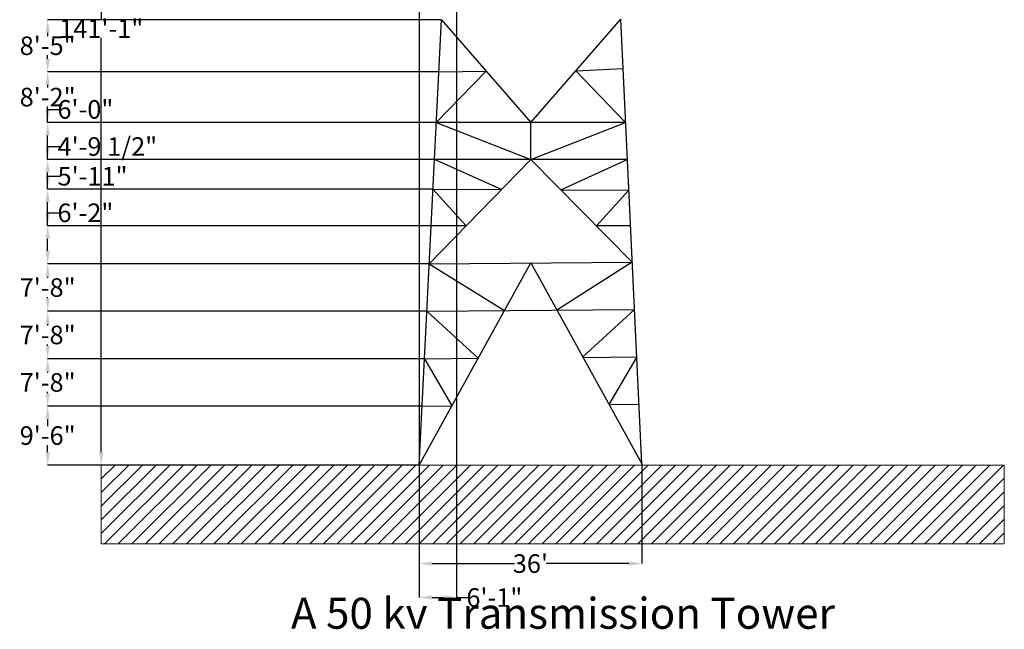
# Model space of a CAD drawing. Units: inches. Extents: x -827 to 1185, y -311 to 1858.
# Tile 1 of 2: x -754 to 1156, y -311 to 871. Entities that reach past the tile are written whole.
import ezdxf

# ---------------------------------------------------------------- set-up
doc = ezdxf.new("R2010")
doc.units = ezdxf.units.IN
doc.header["$MEASUREMENT"] = 0
for name, color, linetype, lineweight in [('C-TOPO-PATT', 8, 'Continuous', 18), ('S-ANNO-DIMS', 2, 'Continuous', 18), ('S-ANNO-TEXT', 7, 'Continuous', 25), ('S-TOWR', 5, 'Continuous', 30)]:
    doc.layers.add(name, color=color, linetype=linetype, lineweight=lineweight)
doc.styles.get("Standard").update_dxf_attribs({"font": 'arial.ttf'})
doc.dimstyles.get("Standard").update_dxf_attribs({"dimtxt": 36, "dimasz": 25.18, "dimexe": 0.18, "dimexo": 0.0625, "dimgap": 0.09, "dimtad": 0, "dimtih": 1, "dimtoh": 1, "dimdec": 0, "dimzin": 0, "dimdsep": 46, "dimlunit": 3, "dimtxsty": 'Standard', "dimcen": 0.09, "dimclrd": 4, "dimadec": 0, "dimazin": 0, "dimtfac": 1, "dimtdec": 0, "dimtofl": 0, "dimtmove": 0, "dimatfit": 3, "dimfxl": 1, "dimtolj": 1, "dimtzin": 0, "dimarcsym": 0})

# ---------------------------------------------------------------- blocks, each defined once
blk = doc.blocks.new('*D1')
at = {"layer": 'Defpoints', "color": 0, "transparency": 16777216}
for p in [(20.6, 7.5), (452.6, 9.7), (452.6, -183.7)]:
    blk.add_point(p, dxfattribs=at)
at = {"layer": 'S-ANNO-DIMS', "color": 0, "lineweight": -2, "transparency": 16777216}
for p, q in [((20.6, 7.4), (20.6, -183.8)), ((452.6, 9.6), (452.6, -183.8)), ((45.8, -183.7), (206, -183.7)), ((427.4, -183.7), (267.2, -183.7))]:
    blk.add_line(p, q, dxfattribs=at)
at = {"layer": 'S-ANNO-DIMS', "color": 0, "transparency": 16777216}
for points in [[(45.8, -179.5), (45.8, -187.9), (20.6, -183.7)], [(427.4, -179.5), (427.4, -187.9), (452.6, -183.7)]]:
    blk.add_solid(points, dxfattribs=at)
at = {"layer": 'S-ANNO-DIMS', "color": 0, "transparency": 16777216, "insert": (236.6, -183.7), "char_height": 36, "attachment_point": 5}
blk.add_mtext("\\A1;36'", dxfattribs=at)
blk = doc.blocks.new('*D6')
at = {"layer": 'Defpoints', "color": 0, "transparency": 16777216}
for p in [(-159.4, 1700.6), (-595.9, 7.5), (20.6, 7.5)]:
    blk.add_point(p, dxfattribs=at)
at = {"layer": 'S-ANNO-DIMS', "color": 0, "lineweight": -2, "transparency": 16777216}
for p, q in [((-159.5, 1700.6), (-596.1, 1700.6)), ((-595.9, 1675.4), (-595.9, 872.2)), ((-595.9, 32.6), (-595.9, 835.9)), ((20.5, 7.5), (-596.1, 7.5))]:
    blk.add_line(p, q, dxfattribs=at)
at = {"layer": 'S-ANNO-DIMS', "color": 0, "transparency": 16777216}
for points in [[(-600.1, 1675.4), (-591.7, 1675.4), (-595.9, 1700.6)], [(-600.1, 32.6), (-591.7, 32.6), (-595.9, 7.5)]]:
    blk.add_solid(points, dxfattribs=at)
at = {"layer": 'S-ANNO-DIMS', "color": 0, "transparency": 16777216, "insert": (-595.9, 854), "char_height": 36, "attachment_point": 5}
blk.add_mtext('\\A1;141\'-1"', dxfattribs=at)
blk = doc.blocks.new('*D15')
at = {"layer": 'Defpoints', "color": 0, "transparency": 16777216}
for p in [(-699.9, 121.7), (26.3, 121.7), (20.6, 7.5)]:
    blk.add_point(p, dxfattribs=at)
at = {"layer": 'S-ANNO-DIMS', "color": 0, "lineweight": -2, "transparency": 16777216}
for p, q in [((26.2, 121.7), (-700.1, 121.7)), ((20.5, 7.5), (-700.1, 7.5))]:
    blk.add_line(p, q, dxfattribs=at)
at = {"layer": 'S-ANNO-DIMS', "color": 4, "lineweight": -2, "transparency": 16777216}
for p, q in [((-699.9, 96.5), (-699.9, 83)), ((-699.9, 32.6), (-699.9, 46.1))]:
    blk.add_line(p, q, dxfattribs=at)
at = {"layer": 'S-ANNO-DIMS', "color": 4, "transparency": 16777216}
for points in [[(-704.1, 96.5), (-695.7, 96.5), (-699.9, 121.7)], [(-704.1, 32.6), (-695.7, 32.6), (-699.9, 7.5)]]:
    blk.add_solid(points, dxfattribs=at)
at = {"layer": 'S-ANNO-DIMS', "color": 0, "transparency": 16777216, "insert": (-699.9, 64.6), "char_height": 36, "attachment_point": 5}
blk.add_mtext('\\A1;9\'-6"', dxfattribs=at)
blk = doc.blocks.new('*D16')
at = {"layer": 'Defpoints', "color": 0, "transparency": 16777216}
for p in [(-699.9, 213.7), (30.9, 213.7), (26.3, 121.7)]:
    blk.add_point(p, dxfattribs=at)
at = {"layer": 'S-ANNO-DIMS', "color": 0, "lineweight": -2, "transparency": 16777216}
for p, q in [((30.9, 213.7), (-700.1, 213.7)), ((26.2, 121.7), (-700.1, 121.7))]:
    blk.add_line(p, q, dxfattribs=at)
at = {"layer": 'S-ANNO-DIMS', "color": 4, "lineweight": -2, "transparency": 16777216}
for p, q in [((-699.9, 188.5), (-699.9, 186.2)), ((-699.9, 146.8), (-699.9, 149.2))]:
    blk.add_line(p, q, dxfattribs=at)
at = {"layer": 'S-ANNO-DIMS', "color": 4, "transparency": 16777216}
for points in [[(-704.1, 188.5), (-695.7, 188.5), (-699.9, 213.7)], [(-704.1, 146.8), (-695.7, 146.8), (-699.9, 121.7)]]:
    blk.add_solid(points, dxfattribs=at)
at = {"layer": 'S-ANNO-DIMS', "color": 0, "transparency": 16777216, "insert": (-699.9, 167.7), "char_height": 36, "attachment_point": 5}
blk.add_mtext('\\A1;7\'-8"', dxfattribs=at)
blk = doc.blocks.new('*D17')
at = {"layer": 'Defpoints', "color": 0, "transparency": 16777216}
for p in [(-699.9, 305.8), (35.5, 305.8), (30.9, 213.7)]:
    blk.add_point(p, dxfattribs=at)
at = {"layer": 'S-ANNO-DIMS', "color": 0, "lineweight": -2, "transparency": 16777216}
for p, q in [((35.5, 305.8), (-700.1, 305.8)), ((30.9, 213.7), (-700.1, 213.7))]:
    blk.add_line(p, q, dxfattribs=at)
at = {"layer": 'S-ANNO-DIMS', "color": 4, "lineweight": -2, "transparency": 16777216}
for p, q in [((-699.9, 280.6), (-699.9, 278.2)), ((-699.9, 238.9), (-699.9, 241.3))]:
    blk.add_line(p, q, dxfattribs=at)
at = {"layer": 'S-ANNO-DIMS', "color": 4, "transparency": 16777216}
for points in [[(-704.1, 280.6), (-695.7, 280.6), (-699.9, 305.8)], [(-704.1, 238.9), (-695.7, 238.9), (-699.9, 213.7)]]:
    blk.add_solid(points, dxfattribs=at)
at = {"layer": 'S-ANNO-DIMS', "color": 0, "transparency": 16777216, "insert": (-699.9, 259.8), "char_height": 36, "attachment_point": 5}
blk.add_mtext('\\A1;7\'-8"', dxfattribs=at)
blk = doc.blocks.new('*D18')
at = {"layer": 'Defpoints', "color": 0, "transparency": 16777216}
for p in [(-699.9, 397.8), (40.2, 397.8), (35.5, 305.8)]:
    blk.add_point(p, dxfattribs=at)
at = {"layer": 'S-ANNO-DIMS', "color": 0, "lineweight": -2, "transparency": 16777216}
for p, q in [((40.1, 397.8), (-700.1, 397.8)), ((35.5, 305.8), (-700.1, 305.8))]:
    blk.add_line(p, q, dxfattribs=at)
at = {"layer": 'S-ANNO-DIMS', "color": 4, "lineweight": -2, "transparency": 16777216}
for p, q in [((-699.9, 372.7), (-699.9, 370.3)), ((-699.9, 331), (-699.9, 333.3))]:
    blk.add_line(p, q, dxfattribs=at)
at = {"layer": 'S-ANNO-DIMS', "color": 4, "transparency": 16777216}
for points in [[(-704.1, 372.7), (-695.7, 372.7), (-699.9, 397.8)], [(-704.1, 331), (-695.7, 331), (-699.9, 305.8)]]:
    blk.add_solid(points, dxfattribs=at)
at = {"layer": 'S-ANNO-DIMS', "color": 0, "transparency": 16777216, "insert": (-699.9, 351.8), "char_height": 36, "attachment_point": 5}
blk.add_mtext('\\A1;7\'-8"', dxfattribs=at)
blk = doc.blocks.new('*D19')
at = {"layer": 'Defpoints', "color": 0, "transparency": 16777216}
for p in [(-699.9, 471.6), (44.9, 471.6), (40.2, 397.8)]:
    blk.add_point(p, dxfattribs=at)
at = {"layer": 'S-ANNO-DIMS', "color": 4, "lineweight": -2, "transparency": 16777216}
for p, q in [((-699.9, 471.6), (-699.9, 496.8)), ((-699.9, 496.8), (-674.7, 496.8)), ((-699.9, 423), (-699.9, 446.5))]:
    blk.add_line(p, q, dxfattribs=at)
at = {"layer": 'S-ANNO-DIMS', "color": 0, "lineweight": -2, "transparency": 16777216}
for p, q in [((44.8, 471.6), (-700.1, 471.6)), ((40.1, 397.8), (-700.1, 397.8))]:
    blk.add_line(p, q, dxfattribs=at)
at = {"layer": 'S-ANNO-DIMS', "color": 4, "transparency": 16777216}
for points in [[(-704.1, 446.5), (-695.7, 446.5), (-699.9, 471.6)], [(-704.1, 423), (-695.7, 423), (-699.9, 397.8)]]:
    blk.add_solid(points, dxfattribs=at)
at = {"layer": 'S-ANNO-DIMS', "color": 0, "transparency": 16777216, "insert": (-626.7, 496.8), "char_height": 36, "attachment_point": 5}
blk.add_mtext('\\A1;6\'-2"', dxfattribs=at)
blk = doc.blocks.new('*D20')
at = {"layer": 'Defpoints', "color": 0, "transparency": 16777216}
for p in [(-699.9, 542.5), (47.4, 542.5), (44.9, 471.6)]:
    blk.add_point(p, dxfattribs=at)
at = {"layer": 'S-ANNO-DIMS', "color": 4, "lineweight": -2, "transparency": 16777216}
for p, q in [((-699.9, 542.5), (-699.9, 567.7)), ((-699.9, 567.7), (-674.7, 567.7)), ((-699.9, 496.8), (-699.9, 517.3))]:
    blk.add_line(p, q, dxfattribs=at)
at = {"layer": 'S-ANNO-DIMS', "color": 0, "lineweight": -2, "transparency": 16777216}
for p, q in [((47.4, 542.5), (-700.1, 542.5)), ((44.8, 471.6), (-700.1, 471.6))]:
    blk.add_line(p, q, dxfattribs=at)
at = {"layer": 'S-ANNO-DIMS', "color": 4, "transparency": 16777216}
for points in [[(-704.1, 517.3), (-695.7, 517.3), (-699.9, 542.5)], [(-704.1, 496.8), (-695.7, 496.8), (-699.9, 471.6)]]:
    blk.add_solid(points, dxfattribs=at)
at = {"layer": 'S-ANNO-DIMS', "color": 0, "transparency": 16777216, "insert": (-612.8, 567.7), "char_height": 36, "attachment_point": 5}
blk.add_mtext('\\A1;5\'-11"', dxfattribs=at)
blk = doc.blocks.new('*D21')
at = {"layer": 'Defpoints', "color": 0, "transparency": 16777216}
for p in [(-699.9, 600.2), (50.9, 600.2), (47.4, 542.5)]:
    blk.add_point(p, dxfattribs=at)
at = {"layer": 'S-ANNO-DIMS', "color": 4, "lineweight": -2, "transparency": 16777216}
for p, q in [((-699.9, 600.2), (-699.9, 625.3)), ((-699.9, 625.3), (-674.7, 625.3)), ((-699.9, 567.7), (-699.9, 575))]:
    blk.add_line(p, q, dxfattribs=at)
at = {"layer": 'S-ANNO-DIMS', "color": 0, "lineweight": -2, "transparency": 16777216}
for p, q in [((50.8, 600.2), (-700.1, 600.2)), ((47.4, 542.5), (-700.1, 542.5))]:
    blk.add_line(p, q, dxfattribs=at)
at = {"layer": 'S-ANNO-DIMS', "color": 4, "transparency": 16777216}
for points in [[(-704.1, 575), (-695.7, 575), (-699.9, 600.2)], [(-704.1, 567.7), (-695.7, 567.7), (-699.9, 542.5)]]:
    blk.add_solid(points, dxfattribs=at)
at = {"layer": 'S-ANNO-DIMS', "color": 0, "transparency": 16777216, "insert": (-584.1, 625.3), "char_height": 36, "attachment_point": 5}
blk.add_mtext('\\A1;4\'-9 1/2"', dxfattribs=at)
blk = doc.blocks.new('*D22')
at = {"layer": 'Defpoints', "color": 0, "transparency": 16777216}
for p in [(-699.9, 672.2), (53.9, 672.2), (50.9, 600.2)]:
    blk.add_point(p, dxfattribs=at)
at = {"layer": 'S-ANNO-DIMS', "color": 4, "lineweight": -2, "transparency": 16777216}
for p, q in [((-699.9, 672.2), (-699.9, 697.4)), ((-699.9, 697.4), (-674.7, 697.4)), ((-699.9, 625.3), (-699.9, 647))]:
    blk.add_line(p, q, dxfattribs=at)
at = {"layer": 'S-ANNO-DIMS', "color": 0, "lineweight": -2, "transparency": 16777216}
for p, q in [((53.9, 672.2), (-700.1, 672.2)), ((50.8, 600.2), (-700.1, 600.2))]:
    blk.add_line(p, q, dxfattribs=at)
at = {"layer": 'S-ANNO-DIMS', "color": 4, "transparency": 16777216}
for points in [[(-704.1, 647), (-695.7, 647), (-699.9, 672.2)], [(-704.1, 625.3), (-695.7, 625.3), (-699.9, 600.2)]]:
    blk.add_solid(points, dxfattribs=at)
at = {"layer": 'S-ANNO-DIMS', "color": 0, "transparency": 16777216, "insert": (-626.7, 697.4), "char_height": 36, "attachment_point": 5}
blk.add_mtext('\\A1;6\'-0"', dxfattribs=at)
blk = doc.blocks.new('*D23')
at = {"layer": 'Defpoints', "color": 0, "transparency": 16777216}
for p in [(-699.9, 770.1), (58.8, 770.1), (53.9, 672.2)]:
    blk.add_point(p, dxfattribs=at)
at = {"layer": 'S-ANNO-DIMS', "color": 0, "lineweight": -2, "transparency": 16777216}
for p, q in [((58.8, 770.1), (-700.1, 770.1)), ((53.9, 672.2), (-700.1, 672.2))]:
    blk.add_line(p, q, dxfattribs=at)
at = {"layer": 'S-ANNO-DIMS', "color": 4, "lineweight": -2, "transparency": 16777216}
for p, q in [((-699.9, 745), (-699.9, 739.7)), ((-699.9, 697.4), (-699.9, 702.7))]:
    blk.add_line(p, q, dxfattribs=at)
at = {"layer": 'S-ANNO-DIMS', "color": 4, "transparency": 16777216}
for points in [[(-704.1, 745), (-695.7, 745), (-699.9, 770.1)], [(-704.1, 697.4), (-695.7, 697.4), (-699.9, 672.2)]]:
    blk.add_solid(points, dxfattribs=at)
at = {"layer": 'S-ANNO-DIMS', "color": 0, "transparency": 16777216, "insert": (-699.9, 721.2), "char_height": 36, "attachment_point": 5}
blk.add_mtext('\\A1;8\'-2"', dxfattribs=at)
blk = doc.blocks.new('*D24')
at = {"layer": 'Defpoints', "color": 0, "transparency": 16777216}
for p in [(-699.9, 871.4), (63.9, 871.4), (58.8, 770.1)]:
    blk.add_point(p, dxfattribs=at)
at = {"layer": 'S-ANNO-DIMS', "color": 0, "lineweight": -2, "transparency": 16777216}
for p, q in [((63.8, 871.4), (-700.1, 871.4)), ((58.8, 770.1), (-700.1, 770.1))]:
    blk.add_line(p, q, dxfattribs=at)
at = {"layer": 'S-ANNO-DIMS', "color": 4, "lineweight": -2, "transparency": 16777216}
for p, q in [((-699.9, 846.2), (-699.9, 839.2)), ((-699.9, 795.3), (-699.9, 802.3))]:
    blk.add_line(p, q, dxfattribs=at)
at = {"layer": 'S-ANNO-DIMS', "color": 4, "transparency": 16777216}
for points in [[(-704.1, 846.2), (-695.7, 846.2), (-699.9, 871.4)], [(-704.1, 795.3), (-695.7, 795.3), (-699.9, 770.1)]]:
    blk.add_solid(points, dxfattribs=at)
at = {"layer": 'S-ANNO-DIMS', "color": 0, "transparency": 16777216, "insert": (-699.9, 820.8), "char_height": 36, "attachment_point": 5}
blk.add_mtext('\\A1;8\'-5"', dxfattribs=at)
blk = doc.blocks.new('*D33')
at = {"layer": 'Defpoints', "color": 0, "transparency": 16777216}
for p in [(20.6, 1496.6), (93.5, 1496.6), (93.5, -249.5)]:
    blk.add_point(p, dxfattribs=at)
at = {"layer": 'S-ANNO-DIMS', "color": 0, "lineweight": -2, "transparency": 16777216}
for p, q in [((20.6, 1496.5), (20.6, -249.7)), ((93.5, 1496.5), (93.5, -249.7))]:
    blk.add_line(p, q, dxfattribs=at)
at = {"layer": 'S-ANNO-DIMS', "color": 4, "lineweight": -2, "transparency": 16777216}
for p, q in [((45.8, -249.5), (68.3, -249.5)), ((93.5, -249.5), (118.7, -249.5))]:
    blk.add_line(p, q, dxfattribs=at)
at = {"layer": 'S-ANNO-DIMS', "color": 4, "transparency": 16777216}
for points in [[(45.8, -245.3), (45.8, -253.7), (20.6, -249.5)], [(68.3, -245.3), (68.3, -253.7), (93.5, -249.5)]]:
    blk.add_solid(points, dxfattribs=at)
at = {"layer": 'S-ANNO-DIMS', "color": 0, "transparency": 16777216, "insert": (166.7, -249.5), "char_height": 36, "attachment_point": 5}
blk.add_mtext('\\A1;6\'-1"', dxfattribs=at)

msp = doc.modelspace()

# ---------------------------------------------------------------- hatches: boundary and pattern name
at = {"layer": 'C-TOPO-PATT'}
h = msp.add_hatch(dxfattribs=at)
h.set_pattern_fill('ANSI31', color=256, scale=150, style=0)
h.set_pattern_definition([(45, (-1783.912, -146.804), (-13.25825, 13.25825), [])])
h.paths.add_polyline_path([(-595.91, 7.45), (1155.95, 7.45), (1155.95, -145.49), (-595.91, -145.49)])

# ---------------------------------------------------------------- linework, layer by layer
msp.add_lwpolyline([(-595.91, 7.45), (1155.95, 7.45), (1155.95, -145.49), (-595.91, -145.49)], close=True, dxfattribs=at)
at = {"layer": 'S-TOWR'}
for p, q in [((20.58, 7.45), (63.91, 871.37)), ((63.91, 871.37), (237.6, 672.23)), ((237.6, 672.23), (411.9, 872.2)), ((452.58, 9.7), (411.9, 872.2)), ((53.92, 672.23), (150.75, 771.8)), ((58.83, 770.15), (150.75, 771.8)), ((324.37, 772.06), (324.11, 772.06)), ((324.37, 772.06), (324.24, 772.21)), ((324.75, 772.22), (416.41, 776.54)), ((421.33, 672.23), (324.75, 772.22)), ((421.33, 672.23), (53.92, 672.23)), ((53.92, 672.23), (237.51, 600.15)), ((236.58, 672.23), (238, 672.69)), ((239.29, 672.25), (236.58, 672.23)), ((237.48, 672.24), (238.38, 672.24)), ((237.49, 600.15), (237.6, 672.56)), ((237.51, 600.15), (421.33, 672.23)), ((237.49, 600.15), (40.16, 397.85)), ((424.11, 600.15), (50.87, 600.15)), ((181.61, 541.24), (50.87, 600.15)), ((237.49, 600.16), (434.11, 401.2)), ((295.71, 541.24), (424.11, 600.15)), ((47.42, 542.5), (47.38, 542.26)), ((47.38, 542.26), (47.41, 542.26)), ((112.14, 471.64), (47.42, 542.5)), ((47.42, 542.5), (180.6, 541.83)), ((295.71, 541.24), (427.54, 540.58)), ((427.54, 540.58), (364.5, 471.64)), ((427.06, 541.38), (426.99, 541.38)), ((112.14, 471.64), (44.87, 471.64)), ((429.78, 471.64), (364.5, 471.64)), ((40.16, 397.85), (434.11, 401.2)), ((434.11, 401.2), (287.79, 307.93)), ((20.58, 7.45), (237.18, 399.52)), ((40.16, 397.85), (186.1, 307.06)), ((237.18, 399.52), (452.58, 9.7)), ((35.55, 305.78), (438.45, 309.21)), ((35.55, 305.78), (135.02, 214.6)), ((438.45, 309.21), (337.82, 216.67)), ((30.93, 213.72), (135.02, 214.6)), ((30.93, 213.72), (83.94, 122.14)), ((338.4, 216.33), (442.79, 217.22)), ((442.79, 217.22), (389.01, 124.74)), ((26.31, 121.65), (83.94, 122.14)), ((389.01, 124.74), (447.13, 125.23))]:
    msp.add_line(p, q, dxfattribs=at)

# ---------------------------------------------------------------- texts
at = {"layer": 'S-ANNO-TEXT', "insert": (-227.93, -250.13), "char_height": 60, "attachment_point": 1}
msp.add_mtext_dynamic_manual_height_columns('{A 50 kv Transmission Tower}', width=1214.4183, gutter_width=1, heights=[0], dxfattribs=at)

# ---------------------------------------------------------------- dimensions: what is measured, and where the dimension line sits
at = {"layer": 'S-ANNO-DIMS'}
for base, p1, p2, override, picture, middle in [((-595.91, 7.45), (-159.42, 1700.58), (20.58, 7.45), {"dimclrd": 0, "dimclre": 0, "dimclrt": 0}, '*D6', (-595.91, 854.01)), ((-699.91, 871.37), (58.83, 770.15), (63.91, 871.37), {"dimdec": 1, "dimlfac": 1, "dimrnd": 0, "dimzin": 1, "dimdsep": 46, "dimlunit": 4, "dimfrac": 2}, '*D24', (-699.91, 820.76)), ((-699.91, 770.15), (53.92, 672.23), (58.83, 770.15), {"dimdec": 1, "dimlfac": 1, "dimrnd": 0, "dimzin": 1, "dimdsep": 46, "dimlunit": 4, "dimfrac": 2}, '*D23', (-699.91, 721.19)), ((-699.91, 672.23), (50.87, 600.15), (53.92, 672.23), {"dimdec": 1, "dimlfac": 1, "dimrnd": 0, "dimzin": 1, "dimdsep": 46, "dimlunit": 4, "dimfrac": 2}, '*D22', (-626.7, 697.41)), ((-699.9144, 600.1522), (47.4176, 542.5024), (50.872, 600.1522), {"dimdec": 1, "dimlfac": 1, "dimrnd": 0, "dimzin": 1, "dimdsep": 46, "dimlunit": 4, "dimfrac": 2}, '*D21', (-584.1287, 625.3322)), ((-699.91, 542.5), (44.87, 471.64), (47.42, 542.5), {"dimdec": 1, "dimlfac": 1, "dimrnd": 0, "dimzin": 1, "dimdsep": 46, "dimlunit": 4, "dimfrac": 2}, '*D20', (-612.81, 567.68)), ((-699.91, 471.64), (40.16, 397.85), (44.87, 471.64), {"dimdec": 1, "dimlfac": 1, "dimrnd": 0, "dimzin": 1, "dimdsep": 46, "dimlunit": 4, "dimfrac": 2}, '*D19', (-626.7, 496.82)), ((-699.91, 397.85), (35.55, 305.78), (40.16, 397.85), {"dimdec": 1, "dimlfac": 1, "dimrnd": 0, "dimzin": 1, "dimdsep": 46, "dimlunit": 4, "dimfrac": 2}, '*D18', (-699.91, 351.81)), ((-699.91, 305.78), (30.93, 213.72), (35.55, 305.78), {"dimdec": 1, "dimlfac": 1, "dimrnd": 0, "dimzin": 1, "dimdsep": 46, "dimlunit": 4, "dimfrac": 2}, '*D17', (-699.91, 259.75)), ((-699.91, 213.72), (26.31, 121.65), (30.93, 213.72), {"dimdec": 1, "dimlfac": 1, "dimrnd": 0, "dimzin": 1, "dimdsep": 46, "dimlunit": 4, "dimfrac": 2}, '*D16', (-699.91, 167.69)), ((-699.91, 121.65), (20.58, 7.45), (26.31, 121.65), {"dimdec": 1, "dimlfac": 1, "dimrnd": 0, "dimzin": 1, "dimdsep": 46, "dimlunit": 4, "dimfrac": 2}, '*D15', (-699.91, 64.55))]:
    dim = msp.add_linear_dim(base=base, p1=p1, p2=p2, angle=90, dimstyle='Standard', override=override, dxfattribs=at)
    dim.commit()
    dim.dimension.update_dxf_attribs({"geometry": picture, "text_midpoint": middle})
for base, p1, p2, override, picture, middle in [((93.47, -249.49), (20.58, 1496.58), (93.47, 1496.58), {"dimdec": 1, "dimlfac": 1, "dimrnd": 0, "dimzin": 1, "dimdsep": 46, "dimlunit": 4, "dimfrac": 2}, '*D33', (166.69, -249.49)), ((452.58, -183.67), (20.58, 7.45), (452.58, 9.7), {"dimclrd": 0, "dimclre": 0, "dimclrt": 0}, '*D1', (236.58, -183.67))]:
    dim = msp.add_linear_dim(base=base, p1=p1, p2=p2, dimstyle='Standard', override=override, dxfattribs=at)
    dim.commit()
    dim.dimension.update_dxf_attribs({"geometry": picture, "text_midpoint": middle})

doc.saveas('drawing.dxf')
